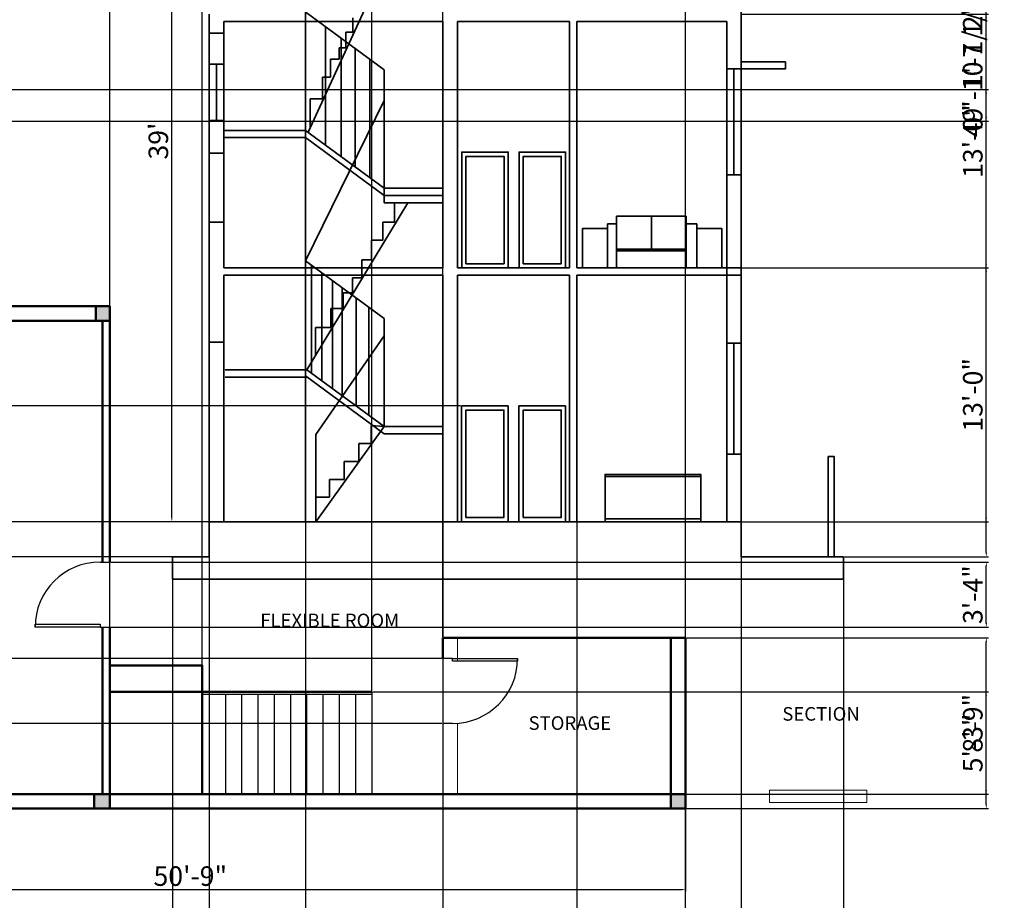
# Model space of a CAD drawing. Units: inches. Extents: x 1367 to 2309, y 1406 to 3826.
# Tile 8 of 9: x 1704 to 2309, y 2918 to 3460. Entities that reach past the tile are written whole.
import ezdxf

# ---------------------------------------------------------------- set-up
doc = ezdxf.new("R2010")
doc.units = ezdxf.units.IN
for name, color, linetype, lineweight in [('A-ANNO-DIMS', 2, 'Continuous', 18), ('A-ANNO-TEXT', 7, 'Continuous', 25), ('A-AREA-IDEN', 3, 'Continuous', 18), ('A-DOOR', 4, 'Continuous', 25), ('A-FLOR-STRS', 7, 'Continuous', 25), ('A-FURN', 8, 'Continuous', 18), ('A-SECT', 7, 'Continuous', 35), ('A-WALL', 7, 'Continuous', 50), ('A-WALL-PATT', 8, 'Continuous', 18)]:
    doc.layers.add(name, color=color, linetype=linetype, lineweight=lineweight)
doc.styles.get("Standard").update_dxf_attribs({"font": 'arial.ttf'})
doc.dimstyles.new('ISO-25', dxfattribs={"dimtxt": 12, "dimasz": 2.5, "dimexe": 1.25, "dimexo": 0.625, "dimtad": 1, "dimdec": 0, "dimlunit": 4, "dimtxsty": 'Standard', "dimcen": 2.5, "dimadec": 0, "dimazin": 0, "dimtfac": 1, "dimtdec": 0, "dimtmove": 0, "dimatfit": 3, "dimfxl": 1, "dimarcsym": 0})

# ---------------------------------------------------------------- blocks, each defined once
blk = doc.blocks.new('*U2')
for p, q in [((0, 0), (0, -6)), ((40, 0), (40, -6))]:
    blk.add_line(p, q)
blk.add_lwpolyline([(0, 0), (0, 40), (1.75, 40), (1.75, 0)], close=True)
blk.add_arc((0, 0), 40, 0, 90)
blk = doc.blocks.new('*D39')
at = {"layer": 'A-ANNO-DIMS', "color": 0, "lineweight": -2, "transparency": 16777216}
for p, q in [((1504.37, 2973.99), (1504.37, 2923.6)), ((2113.4, 2973.99), (2113.4, 2923.6)), ((1506.87, 2924.85), (2110.9, 2924.85))]:
    blk.add_line(p, q, dxfattribs=at)
at = {"layer": 'A-ANNO-DIMS', "color": 0, "lineweight": 100, "transparency": 16777216}
for points in [[(1506.87, 2925.27), (1506.87, 2924.44), (1504.37, 2924.85)], [(2110.9, 2925.27), (2110.9, 2924.44), (2113.4, 2924.85)]]:
    blk.add_solid(points, dxfattribs=at)
at = {"layer": 'Defpoints', "color": 0, "lineweight": 100, "transparency": 16777216}
for p in [(1504.37, 2974.62), (2113.4, 2974.62), (2113.4, 2924.85)]:
    blk.add_point(p, dxfattribs=at)
at = {"layer": 'A-ANNO-DIMS', "color": 0, "transparency": 16777216, "insert": (1808.89, 2931.6), "char_height": 12, "attachment_point": 5}
blk.add_mtext('50\'-9"', dxfattribs=at)
blk = doc.blocks.new('*D42')
at = {"layer": 'A-ANNO-DIMS', "color": 0, "lineweight": -2, "transparency": 16777216}
for p, q in [((1819.79, 3619.06), (1796.28, 3619.06)), ((1797.53, 3153.56), (1797.53, 3616.56)), ((1819.79, 3151.06), (1796.28, 3151.06))]:
    blk.add_line(p, q, dxfattribs=at)
at = {"layer": 'A-ANNO-DIMS', "color": 0, "lineweight": 100, "transparency": 16777216}
for points in [[(1797.12, 3616.56), (1797.95, 3616.56), (1797.53, 3619.06)], [(1797.12, 3153.56), (1797.95, 3153.56), (1797.53, 3151.06)]]:
    blk.add_solid(points, dxfattribs=at)
at = {"layer": 'Defpoints', "color": 0, "lineweight": 100, "transparency": 16777216}
for p in [(1797.53, 3619.06), (1820.42, 3619.06), (1820.42, 3151.06)]:
    blk.add_point(p, dxfattribs=at)
at = {"layer": 'A-ANNO-DIMS', "color": 0, "transparency": 16777216, "insert": (1790.78, 3385.06), "char_height": 12, "attachment_point": 5, "rotation": 90}
blk.add_mtext("39'", dxfattribs=at)
blk = doc.blocks.new('*D87')
at = {"layer": 'A-ANNO-DIMS', "color": 0, "lineweight": -2, "transparency": 16777216}
for p, q in [((1513.37, 2814.79), (1513.37, 3802.6)), ((2113.4, 2814.79), (2113.4, 3802.6)), ((1515.87, 3801.35), (2110.9, 3801.35))]:
    blk.add_line(p, q, dxfattribs=at)
at = {"layer": 'A-ANNO-DIMS', "color": 0, "lineweight": 100, "transparency": 16777216}
for points in [[(1515.87, 3801.77), (1515.87, 3800.93), (1513.37, 3801.35)], [(2110.9, 3801.77), (2110.9, 3800.93), (2113.4, 3801.35)]]:
    blk.add_solid(points, dxfattribs=at)
at = {"layer": 'Defpoints', "color": 0, "lineweight": 100, "transparency": 16777216}
for p in [(2113.4, 3801.35), (1513.37, 2814.17), (2113.4, 2814.17)]:
    blk.add_point(p, dxfattribs=at)
at = {"layer": 'A-ANNO-DIMS', "color": 0, "transparency": 16777216, "insert": (1813.39, 3808.1), "char_height": 12, "attachment_point": 5}
blk.add_mtext('50\'-0"', dxfattribs=at)
blk = doc.blocks.new('*D103')
at = {"layer": 'A-ANNO-DIMS', "color": 0, "lineweight": -2, "transparency": 16777216}
for p, q in [((1504.37, 3284.24), (1504.37, 3802.6)), ((1759.42, 3284.24), (1759.42, 3802.6)), ((1506.87, 3801.35), (1756.92, 3801.35))]:
    blk.add_line(p, q, dxfattribs=at)
at = {"layer": 'A-ANNO-DIMS', "color": 0, "lineweight": 100, "transparency": 16777216}
for points in [[(1506.87, 3801.77), (1506.87, 3800.93), (1504.37, 3801.35)], [(1756.92, 3801.77), (1756.92, 3800.93), (1759.42, 3801.35)]]:
    blk.add_solid(points, dxfattribs=at)
at = {"layer": 'Defpoints', "color": 0, "lineweight": 100, "transparency": 16777216}
for p in [(1759.42, 3801.35), (1504.37, 3283.62), (1759.42, 3283.62)]:
    blk.add_point(p, dxfattribs=at)
at = {"layer": 'A-ANNO-DIMS', "color": 0, "transparency": 16777216, "insert": (1631.89, 3808.1), "char_height": 12, "attachment_point": 5}
blk.add_mtext('21\'-3"', dxfattribs=at)
blk = doc.blocks.new('*D105')
at = {"layer": 'A-ANNO-DIMS', "color": 0, "lineweight": -2, "transparency": 16777216}
for p, q in [((1760.04, 3126.23), (2299.51, 3126.23)), ((2298.26, 3088.73), (2298.26, 3123.73)), ((1760.04, 3086.23), (2299.51, 3086.23))]:
    blk.add_line(p, q, dxfattribs=at)
at = {"layer": 'A-ANNO-DIMS', "color": 0, "lineweight": 100, "transparency": 16777216}
for points in [[(2297.84, 3123.73), (2298.67, 3123.73), (2298.26, 3126.23)], [(2297.84, 3088.73), (2298.67, 3088.73), (2298.26, 3086.23)]]:
    blk.add_solid(points, dxfattribs=at)
at = {"layer": 'Defpoints', "color": 0, "lineweight": 100, "transparency": 16777216}
for p in [(1759.42, 3126.23), (2298.26, 3126.23), (1759.42, 3086.23)]:
    blk.add_point(p, dxfattribs=at)
at = {"layer": 'A-ANNO-DIMS', "color": 0, "transparency": 16777216, "insert": (2291.5, 3106.23), "char_height": 12, "attachment_point": 5, "rotation": 90}
blk.add_mtext('3\'-4"', dxfattribs=at)
blk = doc.blocks.new('*D106')
at = {"layer": 'A-ANNO-DIMS', "color": 0, "lineweight": -2, "transparency": 16777216}
for p, q in [((1759.42, 3063.31), (1759.42, 3802.6)), ((1964.13, 3080.24), (1964.13, 3802.6)), ((1761.92, 3801.35), (1961.63, 3801.35))]:
    blk.add_line(p, q, dxfattribs=at)
at = {"layer": 'A-ANNO-DIMS', "color": 0, "lineweight": 100, "transparency": 16777216}
for points in [[(1761.92, 3801.77), (1761.92, 3800.93), (1759.42, 3801.35)], [(1961.63, 3801.77), (1961.63, 3800.93), (1964.13, 3801.35)]]:
    blk.add_solid(points, dxfattribs=at)
at = {"layer": 'Defpoints', "color": 0, "lineweight": 100, "transparency": 16777216}
for p in [(1964.13, 3801.35), (1964.13, 3079.62), (1759.42, 3062.68)]:
    blk.add_point(p, dxfattribs=at)
at = {"layer": 'A-ANNO-DIMS', "color": 0, "transparency": 16777216, "insert": (1861.77, 3808.18), "char_height": 12, "attachment_point": 5}
blk.add_mtext('17\'-0 1/2"', dxfattribs=at)
blk = doc.blocks.new('*D107')
at = {"layer": 'A-ANNO-DIMS', "color": 0, "lineweight": -2, "transparency": 16777216}
for p, q in [((1964.13, 3080.24), (1964.13, 3802.6)), ((2113.4, 3080.24), (2113.4, 3802.6)), ((1966.63, 3801.35), (2110.9, 3801.35))]:
    blk.add_line(p, q, dxfattribs=at)
at = {"layer": 'A-ANNO-DIMS', "color": 0, "lineweight": 100, "transparency": 16777216}
for points in [[(1966.63, 3801.77), (1966.63, 3800.93), (1964.13, 3801.35)], [(2110.9, 3801.77), (2110.9, 3800.93), (2113.4, 3801.35)]]:
    blk.add_solid(points, dxfattribs=at)
at = {"layer": 'Defpoints', "color": 0, "lineweight": 100, "transparency": 16777216}
for p in [(2113.4, 3801.35), (1964.13, 3079.62), (2113.4, 3079.62)]:
    blk.add_point(p, dxfattribs=at)
at = {"layer": 'A-ANNO-DIMS', "color": 0, "transparency": 16777216, "insert": (2038.76, 3808.18), "char_height": 12, "attachment_point": 5}
blk.add_mtext('12\'-5 1/2"', dxfattribs=at)
blk = doc.blocks.new('*D108')
at = {"layer": 'A-ANNO-DIMS', "color": 0, "lineweight": -2, "transparency": 16777216}
for p, q in [((2114.03, 3079.62), (2299.51, 3079.62)), ((2298.26, 2977.12), (2298.26, 3077.12)), ((2114.03, 2974.62), (2299.51, 2974.62))]:
    blk.add_line(p, q, dxfattribs=at)
at = {"layer": 'A-ANNO-DIMS', "color": 0, "lineweight": 100, "transparency": 16777216}
for points in [[(2297.84, 3077.12), (2298.67, 3077.12), (2298.26, 3079.62)], [(2297.84, 2977.12), (2298.67, 2977.12), (2298.26, 2974.62)]]:
    blk.add_solid(points, dxfattribs=at)
at = {"layer": 'Defpoints', "color": 0, "lineweight": 100, "transparency": 16777216}
for p in [(2113.4, 3079.62), (2298.26, 3079.62), (2113.4, 2974.62)]:
    blk.add_point(p, dxfattribs=at)
at = {"layer": 'A-ANNO-DIMS', "color": 0, "transparency": 16777216, "insert": (2291.51, 3027.12), "char_height": 12, "attachment_point": 5, "rotation": 90}
blk.add_mtext('8\'-9"', dxfattribs=at)
blk = doc.blocks.new('*D109')
at = {"layer": 'A-ANNO-DIMS', "color": 0, "lineweight": -2, "transparency": 16777216}
for p, q in [((1963.5, 3066.97), (1390.27, 3066.97)), ((1391.52, 3029.47), (1391.52, 3064.47)), ((1963.5, 3026.97), (1390.27, 3026.97))]:
    blk.add_line(p, q, dxfattribs=at)
at = {"layer": 'A-ANNO-DIMS', "color": 0, "lineweight": 100, "transparency": 16777216}
for points in [[(1391.1, 3064.47), (1391.94, 3064.47), (1391.52, 3066.97)], [(1391.1, 3029.47), (1391.94, 3029.47), (1391.52, 3026.97)]]:
    blk.add_solid(points, dxfattribs=at)
at = {"layer": 'Defpoints', "color": 0, "lineweight": 100, "transparency": 16777216}
for p in [(1391.52, 3066.97), (1964.13, 3066.97), (1964.13, 3026.97)]:
    blk.add_point(p, dxfattribs=at)
at = {"layer": 'A-ANNO-DIMS', "color": 0, "transparency": 16777216, "insert": (1384.76, 3046.97), "char_height": 12, "attachment_point": 5, "rotation": 90}
blk.add_mtext('3\'-4"', dxfattribs=at)
blk = doc.blocks.new('*D110')
at = {"layer": 'A-ANNO-DIMS', "color": 0, "lineweight": -2, "transparency": 16777216}
for p, q in [((1816.25, 3045.71), (1816.25, 3802.6)), ((1920.42, 3047.12), (1920.42, 3802.6)), ((1818.75, 3801.35), (1917.92, 3801.35))]:
    blk.add_line(p, q, dxfattribs=at)
at = {"layer": 'A-ANNO-DIMS', "color": 0, "lineweight": 100, "transparency": 16777216}
for points in [[(1818.75, 3801.77), (1818.75, 3800.93), (1816.25, 3801.35)], [(1917.92, 3801.77), (1917.92, 3800.93), (1920.42, 3801.35)]]:
    blk.add_solid(points, dxfattribs=at)
at = {"layer": 'Defpoints', "color": 0, "lineweight": 100, "transparency": 16777216}
for p in [(1920.42, 3801.35), (1816.25, 3045.09), (1920.42, 3046.5)]:
    blk.add_point(p, dxfattribs=at)
at = {"layer": 'A-ANNO-DIMS', "color": 0, "transparency": 16777216, "insert": (1868.33, 3808.1), "char_height": 12, "attachment_point": 5}
blk.add_mtext('8\'-8"', dxfattribs=at)
blk = doc.blocks.new('*D111')
at = {"layer": 'A-ANNO-DIMS', "color": 0, "lineweight": -2, "transparency": 16777216}
for p, q in [((1759.42, 3063.31), (1759.42, 3802.6)), ((1816.25, 3063.31), (1816.25, 3802.6)), ((1761.92, 3801.35), (1813.75, 3801.35))]:
    blk.add_line(p, q, dxfattribs=at)
at = {"layer": 'A-ANNO-DIMS', "color": 0, "lineweight": 100, "transparency": 16777216}
for points in [[(1761.92, 3801.77), (1761.92, 3800.93), (1759.42, 3801.35)], [(1813.75, 3801.77), (1813.75, 3800.93), (1816.25, 3801.35)]]:
    blk.add_solid(points, dxfattribs=at)
at = {"layer": 'Defpoints', "color": 0, "lineweight": 100, "transparency": 16777216}
for p in [(1816.25, 3801.35), (1759.42, 3062.68), (1816.25, 3062.68)]:
    blk.add_point(p, dxfattribs=at)
at = {"layer": 'A-ANNO-DIMS', "color": 0, "transparency": 16777216, "insert": (1787.83, 3808.1), "char_height": 12, "attachment_point": 5}
blk.add_mtext('4\'-9"', dxfattribs=at)
blk = doc.blocks.new('*D112')
at = {"layer": 'A-ANNO-DIMS', "color": 0, "lineweight": -2, "transparency": 16777216}
for p, q in [((1921.05, 3046.5), (2299.51, 3046.5)), ((2298.26, 2986.12), (2298.26, 3044)), ((1921.05, 2983.62), (2299.51, 2983.62))]:
    blk.add_line(p, q, dxfattribs=at)
at = {"layer": 'A-ANNO-DIMS', "color": 0, "lineweight": 100, "transparency": 16777216}
for points in [[(2297.84, 3044), (2298.67, 3044), (2298.26, 3046.5)], [(2297.84, 2986.12), (2298.67, 2986.12), (2298.26, 2983.62)]]:
    blk.add_solid(points, dxfattribs=at)
at = {"layer": 'Defpoints', "color": 0, "lineweight": 100, "transparency": 16777216}
for p in [(1920.42, 3046.5), (2298.26, 3046.5), (1920.42, 2983.62)]:
    blk.add_point(p, dxfattribs=at)
at = {"layer": 'A-ANNO-DIMS', "color": 0, "transparency": 16777216, "insert": (2291.5, 3015.06), "char_height": 12, "attachment_point": 5, "rotation": 90}
blk.add_mtext('5\'-3"', dxfattribs=at)
blk = doc.blocks.new('*D113')
at = {"layer": 'A-ANNO-DIMS', "color": 0, "lineweight": -2, "transparency": 16777216}
for p, q in [((1797.9, 3128.9), (1797.9, 2257.28)), ((2210.4, 3128.9), (2210.4, 2257.28)), ((1800.4, 2258.53), (2207.9, 2258.53))]:
    blk.add_line(p, q, dxfattribs=at)
at = {"layer": 'A-ANNO-DIMS', "color": 0, "lineweight": 100, "transparency": 16777216}
for points in [[(1800.4, 2258.94), (1800.4, 2258.11), (1797.9, 2258.53)], [(2207.9, 2258.94), (2207.9, 2258.11), (2210.4, 2258.53)]]:
    blk.add_solid(points, dxfattribs=at)
at = {"layer": 'Defpoints', "color": 0, "lineweight": 100, "transparency": 16777216}
for p in [(1797.9, 3129.52), (2210.4, 3129.52), (2210.4, 2258.53)]:
    blk.add_point(p, dxfattribs=at)
at = {"layer": 'A-ANNO-DIMS', "color": 0, "transparency": 16777216, "insert": (2004.15, 2265.36), "char_height": 12, "attachment_point": 5}
blk.add_mtext('34\'-4 1/2"', dxfattribs=at)
blk = doc.blocks.new('*D114')
at = {"layer": 'A-ANNO-DIMS', "color": 0, "lineweight": -2, "transparency": 16777216}
for p, q in [((1820.42, 3150.44), (1820.42, 2257.28)), ((1879.66, 3150.44), (1879.66, 2257.28)), ((1822.92, 2258.53), (1877.16, 2258.53))]:
    blk.add_line(p, q, dxfattribs=at)
at = {"layer": 'A-ANNO-DIMS', "color": 0, "lineweight": 100, "transparency": 16777216}
for points in [[(1822.92, 2258.94), (1822.92, 2258.11), (1820.42, 2258.53)], [(1877.16, 2258.94), (1877.16, 2258.11), (1879.66, 2258.53)]]:
    blk.add_solid(points, dxfattribs=at)
at = {"layer": 'Defpoints', "color": 0, "lineweight": 100, "transparency": 16777216}
for p in [(1820.42, 3151.06), (1879.66, 3151.06), (1879.66, 2258.53)]:
    blk.add_point(p, dxfattribs=at)
at = {"layer": 'A-ANNO-DIMS', "color": 0, "transparency": 16777216, "insert": (1850.04, 2265.17), "char_height": 12, "attachment_point": 5}
blk.add_mtext('4\'-11"', dxfattribs=at)
blk = doc.blocks.new('*D115')
at = {"layer": 'A-ANNO-DIMS', "color": 0, "lineweight": -2, "transparency": 16777216}
for p, q in [((1879.66, 3150.44), (1879.66, 2257.28)), ((1964.13, 3150.44), (1964.13, 2257.28)), ((1882.16, 2258.53), (1961.63, 2258.53))]:
    blk.add_line(p, q, dxfattribs=at)
at = {"layer": 'A-ANNO-DIMS', "color": 0, "lineweight": 100, "transparency": 16777216}
for points in [[(1882.16, 2258.94), (1882.16, 2258.11), (1879.66, 2258.53)], [(1961.63, 2258.94), (1961.63, 2258.11), (1964.13, 2258.53)]]:
    blk.add_solid(points, dxfattribs=at)
at = {"layer": 'Defpoints', "color": 0, "lineweight": 100, "transparency": 16777216}
for p in [(1879.66, 3151.06), (1964.13, 3151.06), (1964.13, 2258.53)]:
    blk.add_point(p, dxfattribs=at)
at = {"layer": 'A-ANNO-DIMS', "color": 0, "transparency": 16777216, "insert": (1921.89, 2265.35), "char_height": 12, "attachment_point": 5}
blk.add_mtext('7\'-0 1/2"', dxfattribs=at)
blk = doc.blocks.new('*D116')
at = {"layer": 'A-ANNO-DIMS', "color": 0, "lineweight": -2, "transparency": 16777216}
for p, q in [((1964.13, 3150.44), (1964.13, 2257.28)), ((2046.46, 3150.44), (2046.46, 2257.28)), ((1966.63, 2258.53), (2043.96, 2258.53))]:
    blk.add_line(p, q, dxfattribs=at)
at = {"layer": 'A-ANNO-DIMS', "color": 0, "lineweight": 100, "transparency": 16777216}
for points in [[(1966.63, 2258.94), (1966.63, 2258.11), (1964.13, 2258.53)], [(2043.96, 2258.94), (2043.96, 2258.11), (2046.46, 2258.53)]]:
    blk.add_solid(points, dxfattribs=at)
at = {"layer": 'Defpoints', "color": 0, "lineweight": 100, "transparency": 16777216}
for p in [(1964.13, 3151.06), (2046.46, 3151.06), (2046.46, 2258.53)]:
    blk.add_point(p, dxfattribs=at)
at = {"layer": 'A-ANNO-DIMS', "color": 0, "transparency": 16777216, "insert": (2005.29, 2265.35), "char_height": 12, "attachment_point": 5}
blk.add_mtext('6\'-10 1/2"', dxfattribs=at)
blk = doc.blocks.new('*D117')
at = {"layer": 'A-ANNO-DIMS', "color": 0, "lineweight": -2, "transparency": 16777216}
for p, q in [((2046.46, 3150.44), (2046.46, 2257.28)), ((2147.64, 3150.44), (2147.64, 2257.28)), ((2048.96, 2258.53), (2145.14, 2258.53))]:
    blk.add_line(p, q, dxfattribs=at)
at = {"layer": 'A-ANNO-DIMS', "color": 0, "lineweight": 100, "transparency": 16777216}
for points in [[(2048.96, 2258.94), (2048.96, 2258.11), (2046.46, 2258.53)], [(2145.14, 2258.94), (2145.14, 2258.11), (2147.64, 2258.53)]]:
    blk.add_solid(points, dxfattribs=at)
at = {"layer": 'Defpoints', "color": 0, "lineweight": 100, "transparency": 16777216}
for p in [(2046.46, 3151.06), (2147.64, 3151.06), (2147.64, 2258.53)]:
    blk.add_point(p, dxfattribs=at)
at = {"layer": 'A-ANNO-DIMS', "color": 0, "transparency": 16777216, "insert": (2097.05, 2265.28), "char_height": 12, "attachment_point": 5}
blk.add_mtext('8\'-5"', dxfattribs=at)
blk = doc.blocks.new('*D118')
at = {"layer": 'A-ANNO-DIMS', "color": 0, "lineweight": -2, "transparency": 16777216}
for p, q in [((1973.75, 3727.85), (2299.51, 3727.85)), ((2298.26, 3132.02), (2298.26, 3725.35)), ((2211.02, 3129.52), (2299.51, 3129.52))]:
    blk.add_line(p, q, dxfattribs=at)
at = {"layer": 'A-ANNO-DIMS', "color": 0, "lineweight": 100, "transparency": 16777216}
for points in [[(2297.84, 3725.35), (2298.67, 3725.35), (2298.26, 3727.85)], [(2297.84, 3132.02), (2298.67, 3132.02), (2298.26, 3129.52)]]:
    blk.add_solid(points, dxfattribs=at)
at = {"layer": 'Defpoints', "color": 0, "lineweight": 100, "transparency": 16777216}
for p in [(1973.13, 3727.85), (2298.26, 3727.85), (2210.4, 3129.52)]:
    blk.add_point(p, dxfattribs=at)
at = {"layer": 'A-ANNO-DIMS', "color": 0, "transparency": 16777216, "insert": (2291.43, 3428.69), "char_height": 12, "attachment_point": 5, "rotation": 90}
blk.add_mtext('49\'-10 1/2"', dxfattribs=at)
blk = doc.blocks.new('*D119')
at = {"layer": 'A-ANNO-DIMS', "color": 0, "lineweight": -2, "transparency": 16777216}
for p, q in [((2148.26, 3307.06), (2299.51, 3307.06)), ((2298.26, 3153.56), (2298.26, 3304.56)), ((2148.26, 3151.06), (2299.51, 3151.06))]:
    blk.add_line(p, q, dxfattribs=at)
at = {"layer": 'A-ANNO-DIMS', "color": 0, "lineweight": 100, "transparency": 16777216}
for points in [[(2297.84, 3304.56), (2298.67, 3304.56), (2298.26, 3307.06)], [(2297.84, 3153.56), (2298.67, 3153.56), (2298.26, 3151.06)]]:
    blk.add_solid(points, dxfattribs=at)
at = {"layer": 'Defpoints', "color": 0, "lineweight": 100, "transparency": 16777216}
for p in [(2147.64, 3307.06), (2298.26, 3307.06), (2147.64, 3151.06)]:
    blk.add_point(p, dxfattribs=at)
at = {"layer": 'A-ANNO-DIMS', "color": 0, "transparency": 16777216, "insert": (2291.5, 3229.06), "char_height": 12, "attachment_point": 5, "rotation": 90}
blk.add_mtext('13\'-0"', dxfattribs=at)
blk = doc.blocks.new('*D120')
at = {"layer": 'A-ANNO-DIMS', "color": 0, "lineweight": -2, "transparency": 16777216}
for p, q in [((2148.26, 3463.06), (2299.51, 3463.06)), ((2298.26, 3309.56), (2298.26, 3460.56)), ((2148.26, 3307.06), (2299.51, 3307.06))]:
    blk.add_line(p, q, dxfattribs=at)
at = {"layer": 'A-ANNO-DIMS', "color": 0, "lineweight": 100, "transparency": 16777216}
for points in [[(2297.84, 3460.56), (2298.67, 3460.56), (2298.26, 3463.06)], [(2297.84, 3309.56), (2298.67, 3309.56), (2298.26, 3307.06)]]:
    blk.add_solid(points, dxfattribs=at)
at = {"layer": 'Defpoints', "color": 0, "lineweight": 100, "transparency": 16777216}
for p in [(2147.64, 3463.06), (2298.26, 3463.06), (2147.64, 3307.06)]:
    blk.add_point(p, dxfattribs=at)
at = {"layer": 'A-ANNO-DIMS', "color": 0, "transparency": 16777216, "insert": (2291.5, 3385.06), "char_height": 12, "attachment_point": 5, "rotation": 90}
blk.add_mtext('13\'-0"', dxfattribs=at)
blk = doc.blocks.new('*D124')
at = {"layer": 'A-ANNO-DIMS', "color": 0, "lineweight": -2, "transparency": 16777216}
for p, q in [((1391.52, 3151.06), (1391.52, 3213.55)), ((1819.79, 3151.06), (1390.27, 3151.06)), ((1391.52, 3132.02), (1391.52, 3148.56)), ((1819.79, 3129.52), (1390.27, 3129.52))]:
    blk.add_line(p, q, dxfattribs=at)
at = {"layer": 'A-ANNO-DIMS', "color": 0, "lineweight": 100, "transparency": 16777216}
for points in [[(1391.1, 3148.56), (1391.94, 3148.56), (1391.52, 3151.06)], [(1391.1, 3132.02), (1391.94, 3132.02), (1391.52, 3129.52)]]:
    blk.add_solid(points, dxfattribs=at)
at = {"layer": 'Defpoints', "color": 0, "lineweight": 100, "transparency": 16777216}
for p in [(1391.52, 3151.06), (1820.42, 3151.06), (1820.42, 3129.52)]:
    blk.add_point(p, dxfattribs=at)
at = {"layer": 'A-ANNO-DIMS', "color": 0, "transparency": 16777216, "insert": (1384.69, 3183.56), "char_height": 12, "attachment_point": 5, "rotation": 90}
blk.add_mtext('1\'-9 1/2"', dxfattribs=at)
blk = doc.blocks.new('*D126')
at = {"layer": 'A-ANNO-DIMS', "color": 0, "lineweight": -2, "transparency": 16777216}
for p, q in [((1975.08, 3222.26), (1390.27, 3222.26)), ((1391.52, 3153.56), (1391.52, 3219.76)), ((1975.08, 3151.06), (1390.27, 3151.06))]:
    blk.add_line(p, q, dxfattribs=at)
at = {"layer": 'A-ANNO-DIMS', "color": 0, "lineweight": 100, "transparency": 16777216}
for points in [[(1391.1, 3219.76), (1391.94, 3219.76), (1391.52, 3222.26)], [(1391.1, 3153.56), (1391.94, 3153.56), (1391.52, 3151.06)]]:
    blk.add_solid(points, dxfattribs=at)
at = {"layer": 'Defpoints', "color": 0, "lineweight": 100, "transparency": 16777216}
for p in [(1391.52, 3222.26), (1975.7, 3222.26), (1975.7, 3151.06)]:
    blk.add_point(p, dxfattribs=at)
at = {"layer": 'A-ANNO-DIMS', "color": 0, "transparency": 16777216, "insert": (1384.77, 3186.66), "char_height": 12, "attachment_point": 5, "rotation": 90}
blk.add_mtext('5\'-11"', dxfattribs=at)
blk = doc.blocks.new('*D134')
at = {"layer": 'A-ANNO-DIMS', "color": 0, "lineweight": -2, "transparency": 16777216}
for p, q in [((2298.26, 3416.79), (2298.26, 3479.27)), ((1649.56, 3416.79), (2299.51, 3416.79)), ((2298.26, 3399.83), (2298.26, 3414.29)), ((1649.56, 3397.33), (2299.51, 3397.33))]:
    blk.add_line(p, q, dxfattribs=at)
at = {"layer": 'A-ANNO-DIMS', "color": 0, "lineweight": 100, "transparency": 16777216}
for points in [[(2297.84, 3414.29), (2298.67, 3414.29), (2298.26, 3416.79)], [(2297.84, 3399.83), (2298.67, 3399.83), (2298.26, 3397.33)]]:
    blk.add_solid(points, dxfattribs=at)
at = {"layer": 'Defpoints', "color": 0, "lineweight": 100, "transparency": 16777216}
for p in [(1648.94, 3416.79), (2298.26, 3416.79), (1648.94, 3397.33)]:
    blk.add_point(p, dxfattribs=at)
at = {"layer": 'A-ANNO-DIMS', "color": 0, "transparency": 16777216, "insert": (2291.43, 3449.28), "char_height": 12, "attachment_point": 5, "rotation": 90}
blk.add_mtext('1\'-7 1/2"', dxfattribs=at)

msp = doc.modelspace()

# ---------------------------------------------------------------- hatches: boundary and pattern name
at = {"layer": 'A-WALL-PATT'}
h = msp.add_hatch(color=256, dxfattribs=at)
h.dxf.hatch_style = 1
h.paths.add_polyline_path([(1513.37, 2983.62), (1504.37, 2983.62), (1504.37, 2974.62), (1513.37, 2974.62)])
h.paths.add_polyline_path([(1759.42, 2983.62), (1749.82, 2983.62), (1749.82, 2974.62), (1759.42, 2974.62)])
h.paths.add_polyline_path([(1513.37, 3283.62), (1504.37, 3283.62), (1504.37, 3274.62), (1513.37, 3274.62)])
h.paths.add_polyline_path([(1759.42, 3283.62), (1750.75, 3283.62), (1750.75, 3274.62), (1759.42, 3274.62)])
h.paths.add_polyline_path([(2113.4, 2983.62), (2104.4, 2983.62), (2104.4, 2974.62), (2113.4, 2974.62)])
h.paths.add_polyline_path([(1787.87, 2343.17), (1778.87, 2343.17), (1778.87, 2334.17), (1787.87, 2334.17)])
h.paths.add_polyline_path([(1964.87, 2343.17), (1960.37, 2343.17), (1955.87, 2343.17), (1955.87, 2334.17), (1964.87, 2334.17)])
h.paths.add_polyline_path([(2113.37, 2343.17), (2104.37, 2343.17), (2104.37, 2334.17), (2113.37, 2334.17)])
h.paths.add_polyline_path([(1783.37, 2513.73), (1774.44, 2513.73), (1774.44, 2504.73), (1783.37, 2504.73)])
h.paths.add_polyline_path([(1787.54, 2814.17), (1778.54, 2814.17), (1778.54, 2805.17), (1787.54, 2805.17)])
h.paths.add_polyline_path([(1964.87, 2814.17), (1955.87, 2814.17), (1955.87, 2805.17), (1964.87, 2805.17)])
h.paths.add_polyline_path([(2113.37, 2814.17), (2104.4, 2814.17), (2104.4, 2805.17), (2113.37, 2805.17)])
h.paths.add_polyline_path([(1522.37, 2814.17), (1513.37, 2814.17), (1513.37, 2805.17), (1522.37, 2805.17)])
h.paths.add_polyline_path([(2019.97, 2440.35), (2070.2, 2440.35), (2070.2, 2457.56), (2019.97, 2457.56)], flags=9)
h.paths.add_polyline_path([(1670.17, 2422.1), (1711.32, 2422.1), (1711.32, 2439.31), (1670.17, 2439.31)], flags=9)
h.paths.add_polyline_path([(1917.64, 2783.38), (1946.46, 2783.38), (1946.46, 2800.59), (1917.64, 2800.59)], flags=9)
h.paths.add_polyline_path([(1526.17, 2423.16), (1570.57, 2423.16), (1570.57, 2440.37), (1526.17, 2440.37)], flags=9)
h.paths.add_polyline_path([(2013.98, 2676.57), (2064.21, 2676.57), (2064.21, 2693.79), (2013.98, 2693.79)], flags=9)
h.paths.add_polyline_path([(1738.47, 2785.04), (1767.29, 2785.04), (1767.29, 2802.25), (1738.47, 2802.25)], flags=9)
h.paths.add_polyline_path([(1832.32, 2473.89), (1889.69, 2473.89), (1889.69, 2491.1), (1832.32, 2491.1)], flags=9)
h.paths.add_polyline_path([(1821.9, 2712.75), (1863.05, 2712.75), (1863.05, 2729.96), (1821.9, 2729.96)], flags=9)
h.paths.add_polyline_path([(1595.64, 2683.62), (1684.77, 2683.62), (1684.77, 2700.83), (1595.64, 2700.83)], flags=9)

# ---------------------------------------------------------------- linework, layer by layer
at = {"layer": 'A-FLOR-STRS'}
for p, q in [((1816.25, 3045.09), (1920.42, 3045.09)), ((1830.42, 3045.09), (1830.42, 2983.62)), ((1840.42, 3045.09), (1840.42, 2983.62)), ((1850.42, 3045.09), (1850.42, 2983.62)), ((1860.42, 3045.09), (1860.42, 2983.62)), ((1870.42, 3045.09), (1870.42, 2983.62)), ((1880.42, 3045.09), (1880.42, 2983.62)), ((1890.42, 3045.09), (1890.42, 2983.62)), ((1900.42, 3045.09), (1900.42, 2983.62)), ((1910.42, 3045.09), (1910.42, 2983.62)), ((1920.42, 3046.5), (1920.42, 2983.62))]:
    msp.add_line(p, q, dxfattribs=at)
at = {"layer": 'A-FURN'}
for p, q in [((1973.13, 3065.22), (1973.13, 3079.62)), ((1964.13, 2983.62), (1964.13, 3026.97)), ((1973.13, 2983.62), (1973.13, 3027.08))]:
    msp.add_line(p, q, dxfattribs=at)
msp.add_lwpolyline([(2164.99, 2978.32), (2224.76, 2978.32), (2224.76, 2985.99), (2164.99, 2985.99)], close=True, dxfattribs=at)
at = {"layer": 'A-SECT'}
for p, q in [((1879.66, 3151.06), (1879.66, 3614.56)), ((2147.64, 3579.56), (2147.64, 3454.43)), ((1881.33, 3390.43), (1939.32, 3516.75)), ((1820.42, 3307.06), (1820.42, 3463.06)), ((1880.03, 3464.13), (1928.13, 3428.92)), ((2147.64, 3463.06), (2147.64, 3307.06)), ((1829.42, 3307.06), (1829.42, 3458.56)), ((1829.42, 3458.56), (1964.13, 3458.56)), ((1908.8, 3451.94), (1908.8, 3460.79)), ((1964.13, 3319.85), (1964.13, 3458.56)), ((1973.13, 3315.66), (1973.13, 3458.56)), ((1973.13, 3458.56), (2041.96, 3458.56)), ((2041.96, 3307.06), (2041.96, 3458.56)), ((2046.46, 3458.56), (2138.64, 3458.56)), ((2046.46, 3307.06), (2046.46, 3458.56)), ((2138.64, 3307.06), (2138.64, 3458.56)), ((1891.93, 3382.66), (1891.93, 3455.42)), ((1904.58, 3442.46), (1904.58, 3451.94)), ((1904.58, 3451.94), (1908.8, 3451.94)), ((1901.62, 3375.57), (1901.62, 3448.33)), ((1900.39, 3435.35), (1900.39, 3442.46)), ((1900.39, 3442.46), (1904.58, 3442.46)), ((1910.14, 3369.33), (1910.14, 3442.09)), ((1824.92, 3397.62), (1824.92, 3432.42)), ((1895.14, 3424.36), (1895.14, 3435.35)), ((1895.14, 3435.35), (1900.39, 3435.35)), ((1919.33, 3362.6), (1919.33, 3435.36)), ((1928.13, 3356.16), (1928.13, 3428.92)), ((2143.14, 3429.41), (2143.14, 3364.37)), ((1890.14, 3411.11), (1890.14, 3424.36)), ((1890.14, 3424.36), (1895.14, 3424.36)), ((1928.13, 3409.95), (1879.66, 3311.37)), ((1882.57, 3393.14), (1882.57, 3411.11)), ((1882.57, 3411.11), (1890.14, 3411.11)), ((1829.42, 3391.65), (1879.66, 3391.65)), ((1879.66, 3391.65), (1928.13, 3356.16)), ((1829.42, 3387.15), (1879.66, 3387.15)), ((1879.66, 3387.15), (1928.13, 3351.66)), ((1964.13, 3356.16), (1928.13, 3356.16)), ((1928.13, 3347.16), (1928.13, 3356.16)), ((1964.13, 3351.66), (1928.13, 3351.66)), ((1880.55, 3244.47), (1942.69, 3347.16)), ((1964.13, 3347.16), (1928.13, 3347.16)), ((1934.49, 3335.15), (1934.47, 3347.16)), ((2092.34, 3338.86), (2092.34, 3318.61)), ((1927.22, 3324.17), (1927.22, 3335.15)), ((1927.22, 3335.15), (1934.49, 3335.15)), ((1920.34, 3312.07), (1920.34, 3324.17)), ((1920.34, 3324.17), (1927.22, 3324.17)), ((1964.13, 3307.06), (1964.13, 3319.85)), ((1973.13, 3307.06), (1973.13, 3319.85)), ((2070.94, 3318.61), (2113.73, 3318.61)), ((2070.94, 3317.59), (2113.73, 3317.59)), ((1879.66, 3311.37), (1928.13, 3275.87)), ((1914.26, 3300.87), (1914.26, 3312.07)), ((1914.26, 3312.07), (1920.34, 3312.07)), ((1820.42, 3151.06), (1820.42, 3307.06)), ((1829.42, 3307.06), (1964.13, 3307.06)), ((1883.38, 3242.39), (1883.38, 3308.64)), ((1973.13, 3307.06), (2041.96, 3307.06)), ((2046.46, 3307.06), (2147.64, 3307.06)), ((2138.64, 3151.06), (2138.64, 3307.06)), ((2147.64, 3151.06), (2147.64, 3307.06)), ((1829.42, 3151.06), (1829.42, 3302.56)), ((1829.42, 3302.56), (1964.13, 3302.56)), ((1889.65, 3237.8), (1889.65, 3304.05)), ((1896.25, 3232.97), (1896.25, 3299.21)), ((1908.68, 3291.78), (1908.68, 3300.87)), ((1908.68, 3300.87), (1914.26, 3300.87)), ((1964.13, 3151.06), (1964.13, 3302.56)), ((1973.13, 3151.06), (1973.13, 3302.56)), ((1973.13, 3302.56), (2041.96, 3302.56)), ((2041.96, 3151.06), (2041.96, 3302.56)), ((2046.46, 3151.06), (2046.46, 3302.56)), ((2046.46, 3302.56), (2147.64, 3302.56)), ((1902.34, 3228.51), (1902.34, 3294.76)), ((1902.85, 3282.08), (1902.85, 3291.78)), ((1902.85, 3291.78), (1908.68, 3291.78)), ((1910.8, 3222.31), (1910.8, 3288.56)), ((1895.33, 3270.53), (1895.33, 3282.08)), ((1895.33, 3282.08), (1902.85, 3282.08)), ((1918.67, 3216.55), (1918.67, 3282.8)), ((1879.66, 3275.45), (1879.66, 3151.06)), ((1928.13, 3209.63), (1928.13, 3275.87)), ((1885.83, 3253.2), (1885.83, 3270.53)), ((1885.83, 3270.53), (1895.33, 3270.53)), ((1928.13, 3265.35), (1886.07, 3204.7)), ((2143.14, 3260.77), (2143.14, 3192.49)), ((1879.66, 3245.12), (1928.13, 3209.63)), ((1830.31, 3244.47), (1880.55, 3244.47)), ((1830.31, 3239.97), (1880.55, 3239.97)), ((1879.66, 3240.62), (1928.13, 3205.13)), ((1928.13, 3209.63), (1886.07, 3151.06)), ((1920.16, 3199.09), (1920.16, 3210.09)), ((1920.16, 3210.09), (1928.13, 3209.63)), ((1964.13, 3209.63), (1928.13, 3209.63)), ((1886.07, 3151.06), (1886.07, 3204.7)), ((1964.13, 3205.13), (1928.13, 3205.13)), ((1912.51, 3188.09), (1912.51, 3199.09)), ((1912.51, 3199.09), (1920.16, 3199.09)), ((1903.51, 3177.09), (1903.51, 3188.09)), ((1903.51, 3188.09), (1912.51, 3188.09)), ((2063.93, 3178.76), (2122.65, 3178.76)), ((1894.47, 3166.21), (1894.47, 3177.09)), ((1894.47, 3177.09), (1903.51, 3177.09)), ((1886.07, 3151.06), (1886.07, 3166.21)), ((1886.07, 3166.21), (1894.47, 3166.21)), ((1820.42, 3129.52), (1820.42, 3151.06)), ((1820.42, 3151.06), (2147.64, 3151.06)), ((2063.93, 3152.84), (2122.65, 3152.84)), ((2147.64, 3151.06), (2147.64, 3129.52)), ((1797.9, 3129.52), (1820.42, 3129.52)), ((1797.9, 3129.52), (1797.9, 3115.78)), ((2147.64, 3129.52), (2210.4, 3129.52)), ((2210.4, 3115.78), (2210.4, 3129.52)), ((1797.9, 3115.78), (2210.4, 3115.78))]:
    msp.add_line(p, q, dxfattribs=at)
for points in [[(1820.42, 3377.52), (1829.42, 3377.52), (1829.42, 3451.46), (1820.42, 3451.46)], [(1820.42, 3432.42), (1829.42, 3432.42), (1829.42, 3397.62), (1820.42, 3397.62)], [(2147.64, 3429.41), (2174.74, 3429.41), (2174.74, 3433.75), (2147.64, 3433.75)], [(2138.64, 3429.41), (2147.64, 3429.41), (2147.64, 3364.37), (2138.64, 3364.37)], [(1975.75, 3307.06), (2004.35, 3307.06), (2004.35, 3378.26), (1975.75, 3378.26)], [(2010.98, 3307.06), (2039.57, 3307.06), (2039.57, 3378.26), (2010.98, 3378.26)], [(1978.35, 3309.66), (2001.75, 3309.66), (2001.75, 3375.66), (1978.35, 3375.66)], [(2013.58, 3309.66), (2036.97, 3309.66), (2036.97, 3375.66), (2013.58, 3375.66)], [(2070.94, 3307.06), (2113.73, 3307.06), (2113.73, 3338.86), (2070.94, 3338.86)], [(2050.03, 3307.06), (2065.39, 3307.06), (2065.39, 3331.35), (2050.03, 3331.35)], [(2070.94, 3334.08), (2065.39, 3334.08), (2065.39, 3307.06), (2070.94, 3307.06)], [(2120.31, 3334.08), (2113.73, 3334.13), (2113.73, 3307.11), (2120.31, 3307.06)], [(2120.31, 3307.06), (2135.66, 3307.06), (2135.66, 3331.35), (2120.31, 3331.35)], [(2138.64, 3192.49), (2147.64, 3192.49), (2147.64, 3260.77), (2138.64, 3260.77)], [(1975.7, 3151.06), (2004.3, 3151.06), (2004.3, 3222.26), (1975.7, 3222.26)], [(2010.93, 3151.06), (2039.53, 3151.06), (2039.53, 3222.26), (2010.93, 3222.26)], [(1978.3, 3153.66), (2001.7, 3153.66), (2001.7, 3219.66), (1978.3, 3219.66)], [(2013.53, 3153.66), (2036.93, 3153.66), (2036.93, 3219.66), (2013.53, 3219.66)], [(2201.09, 3129.52), (2204.82, 3129.52), (2204.82, 3191.11), (2201.09, 3191.11)], [(2063.93, 3151.06), (2122.65, 3151.06), (2122.65, 3180.09), (2063.93, 3180.09)]]:
    msp.add_lwpolyline(points, close=True, dxfattribs=at)
msp.add_lwpolyline([(1829.42, 3307.06), (1829.42, 3335.26), (1820.42, 3335.26), (1820.42, 3261.32), (1829.42, 3261.32), (1829.42, 3302.56)], dxfattribs=at)
at = {"layer": 'A-WALL'}
for p, q in [((1504.37, 3283.62), (1759.42, 3283.62)), ((1759.42, 3283.62), (1759.42, 3126.23)), ((1513.37, 3274.62), (1754.92, 3274.62)), ((1754.92, 3274.62), (1754.92, 3126.23)), ((1754.92, 3086.23), (1754.92, 2983.62)), ((1759.42, 3086.23), (1759.42, 2983.62)), ((2113.4, 3079.62), (1964.13, 3079.62)), ((1964.13, 3066.97), (1964.13, 3079.62)), ((2104.4, 2983.62), (2104.4, 3079.62)), ((2113.4, 2983.62), (2113.4, 3079.62)), ((1759.42, 3046.5), (1920.42, 3046.5)), ((1754.92, 2983.62), (1513.37, 2983.62)), ((2113.4, 2983.62), (1759.42, 2983.62)), ((2113.4, 2974.62), (2113.4, 2983.62)), ((1504.37, 2974.62), (2113.4, 2974.62))]:
    msp.add_line(p, q, dxfattribs=at)
for points in [[(1759.42, 3283.62), (1750.75, 3283.62), (1750.75, 3274.62), (1759.42, 3274.62)], [(1759.42, 2983.62), (1816.25, 2983.62), (1816.25, 3062.68), (1759.42, 3062.68)], [(1759.42, 2983.62), (1749.82, 2983.62), (1749.82, 2974.62), (1759.42, 2974.62)], [(2104.4, 2983.62), (2113.4, 2983.62), (2113.4, 2974.62), (2104.4, 2974.62)]]:
    msp.add_lwpolyline(points, close=True, dxfattribs=at)

# ---------------------------------------------------------------- block references
at = {"layer": 'A-DOOR'}
for p, rotation in [((1753.42, 3086.23), 90), ((1970.13, 3066.97), 270)]:
    msp.add_blockref('*U2', p, dxfattribs=dict(at, rotation=rotation))

# ---------------------------------------------------------------- texts
at = {"layer": 'A-ANNO-TEXT', "insert": (2172.85, 3037.07), "char_height": 8.353, "attachment_point": 1}
msp.add_mtext_dynamic_manual_height_columns('SECTION', width=204.251, gutter_width=41.76, heights=[0], dxfattribs=at)
at = {"layer": 'A-AREA-IDEN', "attachment_point": 1}
for s, insert, char_height in [('FLEXIBLE ROOM', (1851.89, 3094.5), 8.3529), ('STORAGE', (2016.83, 3031.43), 8.353)]:
    msp.add_mtext_dynamic_manual_height_columns(s, width=204.251, gutter_width=41.76, heights=[0], dxfattribs=dict(at, insert=insert, char_height=char_height))

# ---------------------------------------------------------------- dimensions: what is measured, and where the dimension line sits
at = {"layer": 'A-ANNO-DIMS'}
for base, p1, p2, override, picture, middle in [((1964.13, 3801.35), (1759.42, 3062.68), (1964.13, 3079.62), {"dimdec": 1, "dimlfac": 1, "dimrnd": 0, "dimzin": 1, "dimdsep": 46, "dimlunit": 4, "dimfrac": 2}, '*D106', (1861.77, 3808.18)), ((2113.4, 3801.35), (1964.13, 3079.62), (2113.4, 3079.62), {"dimdec": 1, "dimlfac": 1, "dimrnd": 0, "dimzin": 1, "dimdsep": 46, "dimlunit": 4, "dimfrac": 2}, '*D107', (2038.76, 3808.18)), ((1759.4169, 3801.349), (1504.3701, 3283.618), (1759.4169, 3283.618), {"dimdec": 1, "dimlfac": 1, "dimrnd": 0, "dimzin": 1, "dimdsep": 46, "dimlunit": 4, "dimfrac": 2}, '*D103', (1631.8935, 3808.105)), ((2113.4, 3801.35), (1513.37, 2814.17), (2113.4, 2814.17), {"dimdec": 1, "dimlfac": 1, "dimrnd": 0, "dimzin": 1, "dimdsep": 46, "dimlunit": 4, "dimfrac": 2}, '*D87', (1813.39, 3808.1)), ((1816.25, 3801.35), (1759.42, 3062.68), (1816.25, 3062.68), {"dimdec": 1, "dimlfac": 1, "dimrnd": 0, "dimzin": 1, "dimdsep": 46, "dimlunit": 4, "dimfrac": 2}, '*D111', (1787.83, 3808.1)), ((1920.42, 3801.35), (1816.25, 3045.09), (1920.42, 3046.5), {"dimdec": 1, "dimlfac": 1, "dimrnd": 0, "dimzin": 1, "dimdsep": 46, "dimlunit": 4, "dimfrac": 2}, '*D110', (1868.33, 3808.1)), ((1879.66, 2258.53), (1820.42, 3151.06), (1879.66, 3151.06), {"dimdec": 1, "dimlfac": 1, "dimrnd": 0, "dimzin": 1, "dimdsep": 46, "dimlunit": 4, "dimfrac": 2}, '*D114', (1850.04, 2265.17)), ((1964.13, 2258.53), (1879.66, 3151.06), (1964.13, 3151.06), {"dimdec": 1, "dimlfac": 1, "dimrnd": 0, "dimzin": 1, "dimdsep": 46, "dimlunit": 4, "dimfrac": 2}, '*D115', (1921.89, 2265.35)), ((2046.46, 2258.53), (1964.13, 3151.06), (2046.46, 3151.06), {"dimdec": 1, "dimlfac": 1, "dimrnd": 0, "dimzin": 1, "dimdsep": 46, "dimlunit": 4, "dimfrac": 2}, '*D116', (2005.29, 2265.35)), ((2147.64, 2258.53), (2046.46, 3151.06), (2147.64, 3151.06), {"dimdec": 1, "dimlfac": 1, "dimrnd": 0, "dimzin": 1, "dimdsep": 46, "dimlunit": 4, "dimfrac": 2}, '*D117', (2097.05, 2265.28)), ((2210.4, 2258.53), (1797.9, 3129.52), (2210.4, 3129.52), {"dimdec": 1, "dimlfac": 1, "dimrnd": 0, "dimzin": 1, "dimdsep": 46, "dimlunit": 4, "dimfrac": 2}, '*D113', (2004.15, 2265.36)), ((2113.4, 2924.85), (1504.37, 2974.62), (2113.4, 2974.62), {"dimclrd": 0, "dimclre": 0, "dimclrt": 0}, '*D39', (1808.89, 2931.6))]:
    dim = msp.add_linear_dim(base=base, p1=p1, p2=p2, dimstyle='ISO-25', override=override, dxfattribs=at)
    dim.commit()
    dim.dimension.update_dxf_attribs({"geometry": picture, "text_midpoint": middle})
for base, p1, p2, override, picture, middle in [((2298.26, 3727.85), (2210.4, 3129.52), (1973.13, 3727.85), {"dimdec": 1, "dimlfac": 1, "dimrnd": 0, "dimzin": 1, "dimdsep": 46, "dimlunit": 4, "dimfrac": 2}, '*D118', (2291.43, 3428.69)), ((1797.53, 3619.06), (1820.42, 3151.06), (1820.42, 3619.06), {"dimclrd": 0, "dimclre": 0, "dimclrt": 0}, '*D42', (1790.78, 3385.06)), ((2298.26, 3416.79), (1648.94, 3397.33), (1648.94, 3416.79), {"dimdec": 1, "dimlfac": 1, "dimrnd": 0, "dimzin": 1, "dimdsep": 46, "dimlunit": 4, "dimfrac": 2}, '*D134', (2291.43, 3449.28)), ((2298.26, 3463.06), (2147.64, 3307.06), (2147.64, 3463.06), {"dimdec": 1, "dimlfac": 1, "dimrnd": 0, "dimzin": 1, "dimdsep": 46, "dimlunit": 4, "dimfrac": 2}, '*D120', (2291.5, 3385.06)), ((2298.26, 3307.06), (2147.64, 3151.06), (2147.64, 3307.06), {"dimdec": 1, "dimlfac": 1, "dimrnd": 0, "dimzin": 1, "dimdsep": 46, "dimlunit": 4, "dimfrac": 2}, '*D119', (2291.5, 3229.06)), ((1391.52, 3222.26), (1975.7, 3151.06), (1975.7, 3222.26), {"dimdec": 1, "dimlfac": 1, "dimrnd": 0, "dimzin": 1, "dimdsep": 46, "dimlunit": 4, "dimfrac": 2}, '*D126', (1384.77, 3186.66)), ((1391.52, 3151.06), (1820.42, 3129.52), (1820.42, 3151.06), {"dimdec": 1, "dimlfac": 1, "dimrnd": 0, "dimzin": 1, "dimdsep": 46, "dimlunit": 4, "dimfrac": 2}, '*D124', (1384.69, 3183.56)), ((2298.26, 3126.23), (1759.42, 3086.23), (1759.42, 3126.23), {"dimdec": 1, "dimlfac": 1, "dimrnd": 0, "dimzin": 1, "dimdsep": 46, "dimlunit": 4, "dimfrac": 2}, '*D105', (2291.5, 3106.23)), ((2298.26, 3079.62), (2113.4, 2974.62), (2113.4, 3079.62), {"dimdec": 1, "dimlfac": 1, "dimrnd": 0, "dimzin": 1, "dimdsep": 46, "dimlunit": 4, "dimfrac": 2}, '*D108', (2291.51, 3027.12)), ((1391.52, 3066.97), (1964.13, 3026.97), (1964.13, 3066.97), {"dimdec": 1, "dimlfac": 1, "dimrnd": 0, "dimzin": 1, "dimdsep": 46, "dimlunit": 4, "dimfrac": 2}, '*D109', (1384.76, 3046.97)), ((2298.26, 3046.5), (1920.42, 2983.62), (1920.42, 3046.5), {"dimdec": 1, "dimlfac": 1, "dimrnd": 0, "dimzin": 1, "dimdsep": 46, "dimlunit": 4, "dimfrac": 2}, '*D112', (2291.5, 3015.06))]:
    dim = msp.add_linear_dim(base=base, p1=p1, p2=p2, angle=90, dimstyle='ISO-25', override=override, dxfattribs=at)
    dim.commit()
    dim.dimension.update_dxf_attribs({"geometry": picture, "text_midpoint": middle})

doc.saveas('drawing.dxf')
